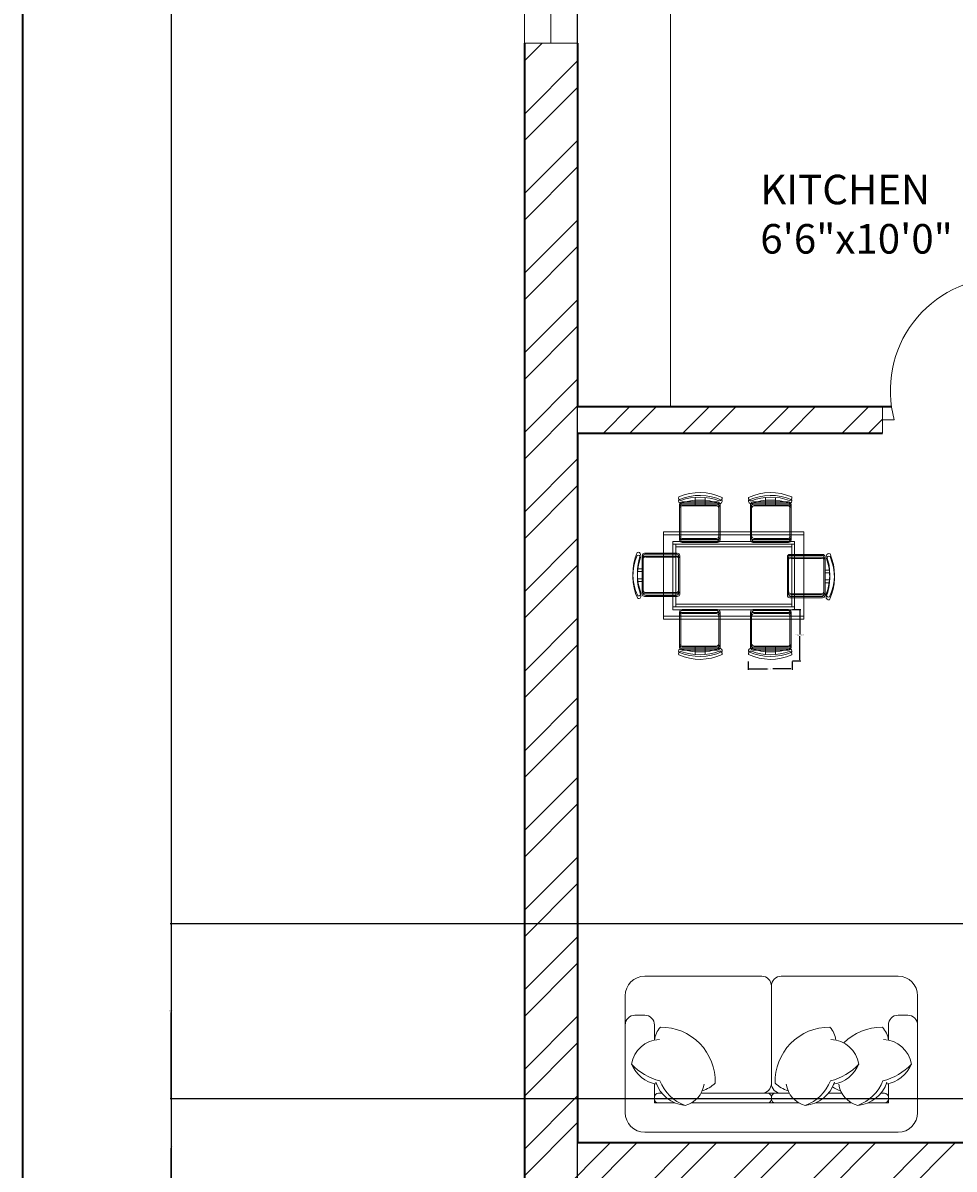
# Model space of a CAD drawing. Units: inches. Extents: x 2552 to 3217, y 1417 to 2737.
# Tile 16 of 25: x 2552 to 2710, y 2392 to 2585. Entities that reach past the tile are written whole.
import ezdxf

# ---------------------------------------------------------------- set-up
doc = ezdxf.new("R2010")
doc.units = ezdxf.units.IN
for name, color, linetype, lineweight in [('A-ANNO-DIMS', 2, 'Continuous', 18), ('A-ANNO-TTLB', 7, 'Continuous', 35), ('A-AREA-IDEN', 7, 'Continuous', 18), ('A-DOOR', 21, 'Continuous', 18), ('A-FLOR-CASE', 9, 'Continuous', 18), ('A-FURN', 8, 'Continuous', 13), ('A-GLAZ', 161, 'Continuous', 18), ('A-WALL', 7, 'Continuous', 35), ('A-WALL-PATT', 217, 'Continuous', 13)]:
    doc.layers.add(name, color=color, linetype=linetype, lineweight=lineweight)
doc.styles.get("Standard").update_dxf_attribs({"font": 'arial.ttf'})
doc.dimstyles.get("Standard").update_dxf_attribs({"dimtxt": 0.18, "dimasz": 0.18, "dimexe": 0.18, "dimexo": 0.0625, "dimgap": 0.09, "dimtad": 0, "dimtih": 1, "dimtoh": 1, "dimdec": 4, "dimzin": 0, "dimdsep": 46, "dimtxsty": 'Standard', "dimcen": 0.09, "dimadec": 0, "dimazin": 0, "dimtfac": 1, "dimtdec": 4, "dimtofl": 0, "dimtmove": 0, "dimatfit": 3, "dimfxl": 1, "dimtolj": 1, "dimtzin": 0, "dimarcsym": 0})

# ---------------------------------------------------------------- blocks, each defined once
blk = doc.blocks.new('TABLE-DINING-RECT')
for points in [[(0, 14.74), (23.77, 14.74), (23.77, 0.48), (0, 0.48)], [(0, 14.74), (23.77, 14.74), (23.77, 0.48), (0, 0.48)], [(0, 14.26), (23.77, 14.26), (23.77, 0), (0, 0)], [(0, 14.26), (23.77, 14.26), (23.77, 0), (0, 0)], [(1.58, 13.15), (22.19, 13.15), (22.19, 2.06), (1.58, 2.06)], [(1.58, 13.15), (22.19, 13.15), (22.19, 2.06), (1.58, 2.06)], [(1.58, 12.68), (22.19, 12.68), (22.19, 1.59), (1.58, 1.59)], [(1.58, 12.68), (22.19, 12.68), (22.19, 1.58), (1.58, 1.58)], [(2.06, 12.68), (21.71, 12.68), (21.71, 2.54), (2.06, 2.54)], [(2.06, 12.68), (21.71, 12.68), (21.71, 2.54), (2.06, 2.54)], [(2.06, 12.2), (21.71, 12.2), (21.71, 2.06), (2.06, 2.06)], [(2.06, 12.2), (21.71, 12.2), (21.71, 2.06), (2.06, 2.06)]]:
    blk.add_lwpolyline(points, close=True)
blk = doc.blocks.new('DINING-CHAIR-NORTH-EAST')
for points in [[(0.51, 7.05, -0.578392), (0.02, 7.59, -0.214524), (7.33, 7.69, -0.552014), (6.98, 7.1, 0.175809), (0.51, 7.05)], [(0.51, 7.05, -0.578392), (0.02, 7.59, -0.214524), (7.33, 7.69, -0.552014), (6.98, 7.1, 0.175809), (0.51, 7.05)], [(0.51, 6.58, -0.578392), (0.02, 7.12, -0.214524), (7.33, 7.22, -0.552014), (6.98, 6.63, 0.175809), (0.51, 6.58)], [(0.51, 6.58, -0.578392), (0.02, 7.12, -0.214524), (7.33, 7.22, -0.552014), (6.98, 6.63, 0.175809), (0.51, 6.58)], [(6.8, 6.84, -0.414214), (7.22, 6.42), (7.22, 0.9, -0.414214), (6.8, 0.48), (0.78, 0.48, -0.414214), (0.36, 0.9), (0.36, 6.42, -0.414214), (0.78, 6.84), (6.8, 6.84)], [(6.8, 6.84, -0.414214), (7.22, 6.42), (7.22, 0.9, -0.414214), (6.8, 0.48), (0.78, 0.48, -0.414214), (0.36, 0.9), (0.36, 6.42, -0.414214), (0.78, 6.84), (6.8, 6.84)], [(6.8, 6.37, -0.414214), (7.22, 5.95), (7.22, 0.42, -0.414214), (6.8, 0), (0.78, 0, -0.414214), (0.36, 0.42), (0.36, 5.95, -0.414214), (0.78, 6.37), (6.8, 6.37)], [(6.8, 6.37, -0.414214), (7.22, 5.95), (7.22, 0.42, -0.414214), (6.8, 0), (0.78, 0, -0.414214), (0.36, 0.42), (0.36, 5.95, -0.414214), (0.78, 6.37), (6.8, 6.37)], [(2.9, 6.84), (2.9, 7.6, 0.064759)], [(2.9, 6.84), (2.9, 7.6, 0.064759)], [(2.9, 6.37), (2.9, 7.13, 0.064759)], [(2.9, 6.37), (2.9, 7.13, 0.064759)]]:
    blk.add_lwpolyline(points, format="xyb")
for points in [[(6.79, 6.65), (0.97, 6.65, 0.414214), (0.55, 6.23), (0.55, 1.09, 0.414214), (0.97, 0.67), (6.79, 0.67, 0.512069), (7.03, 1.09), (7.03, 6.23, 0.512069)], [(6.79, 6.65), (0.97, 6.65, 0.414214), (0.55, 6.23), (0.55, 1.09, 0.414214), (0.97, 0.66), (6.79, 0.66, 0.512069), (7.03, 1.09), (7.03, 6.23, 0.512069)], [(6.79, 6.18), (0.97, 6.18, 0.414214), (0.55, 5.76), (0.55, 0.61, 0.414214), (0.97, 0.19), (6.79, 0.19, 0.512069), (7.03, 0.61), (7.03, 5.76, 0.512069)], [(6.79, 6.18), (0.97, 6.18, 0.414214), (0.55, 5.76), (0.55, 0.61, 0.414214), (0.97, 0.19), (6.79, 0.19, 0.512069), (7.03, 0.61), (7.03, 5.76, 0.512069)]]:
    blk.add_lwpolyline(points, format="xyb", close=True)
for points in [[(4.58, 7.62), (4.58, 6.84)], [(4.58, 7.62), (4.58, 6.84)], [(4.58, 7.14), (4.58, 6.37)], [(4.58, 7.14), (4.58, 6.37)]]:
    blk.add_lwpolyline(points)
blk = doc.blocks.new('DINING-CHAIR-SOUTH-WEST')
for points in [[(6.59, 2.06), (0.58, 2.06, -0.414214), (0.16, 2.48), (0.16, 8.01, -0.414214), (0.58, 8.43), (6.59, 8.43, -0.414214), (7.01, 8.01), (7.01, 2.48, -0.414214), (6.59, 2.06)], [(6.59, 2.06), (0.58, 2.06, -0.414214), (0.16, 2.48), (0.16, 8.01, -0.414214), (0.58, 8.43), (6.59, 8.43, -0.414214), (7.01, 8.01), (7.01, 2.48, -0.414214), (6.59, 2.06)], [(6.59, 1.58), (0.58, 1.58, -0.414214), (0.16, 2), (0.16, 7.53, -0.414214), (0.58, 7.95), (6.59, 7.95, -0.414214), (7.01, 7.53), (7.01, 2, -0.414214), (6.59, 1.58)], [(6.59, 1.58), (0.58, 1.58, -0.414214), (0.16, 2), (0.16, 7.53, -0.414214), (0.58, 7.95), (6.59, 7.95, -0.414214), (7.01, 7.53), (7.01, 2, -0.414214), (6.59, 1.58)], [(4.48, 2.06), (4.48, 1.3, 0.064759)], [(4.48, 2.06), (4.48, 1.3, 0.064759)], [(6.86, 1.85, -0.578392), (7.35, 1.31, -0.214524), (0.05, 1.21, -0.552014), (0.39, 1.8, 0.175809), (6.86, 1.85)], [(6.86, 1.85, -0.578392), (7.35, 1.31, -0.214524), (0.05, 1.21, -0.552014), (0.39, 1.8, 0.175809), (6.86, 1.85)], [(6.86, 1.37, -0.578392), (7.35, 0.83, -0.214524), (0.05, 0.74, -0.552014), (0.39, 1.32, 0.175809), (6.86, 1.37)], [(6.86, 1.37, -0.578392), (7.35, 0.83, -0.214524), (0.05, 0.74, -0.552014), (0.39, 1.32, 0.175809), (6.86, 1.37)], [(4.48, 1.58), (4.48, 0.82, 0.064759)], [(4.48, 1.58), (4.48, 0.82, 0.064759)]]:
    blk.add_lwpolyline(points, format="xyb")
for points in [[(0.58, 2.25), (6.4, 2.25, 0.414214), (6.82, 2.67), (6.82, 7.82, 0.414214), (6.4, 8.24), (0.58, 8.24, 0.512069), (0.35, 7.82), (0.35, 2.67, 0.512069)], [(0.58, 2.25), (6.4, 2.25, 0.414214), (6.82, 2.67), (6.82, 7.82, 0.414214), (6.4, 8.24), (0.58, 8.24, 0.512069), (0.35, 7.82), (0.35, 2.67, 0.512069)], [(0.58, 1.77), (6.4, 1.77, 0.414214), (6.82, 2.19), (6.82, 7.34, 0.414214), (6.4, 7.76), (0.58, 7.76, 0.512069), (0.35, 7.34), (0.35, 2.19, 0.512069)], [(0.58, 1.77), (6.4, 1.77, 0.414214), (6.82, 2.19), (6.82, 7.34, 0.414214), (6.4, 7.76), (0.58, 7.76, 0.512069), (0.35, 7.34), (0.35, 2.19, 0.512069)]]:
    blk.add_lwpolyline(points, format="xyb", close=True)
for points in [[(2.79, 1.28), (2.79, 2.06)], [(2.79, 1.28), (2.79, 2.06)], [(2.79, 0.81), (2.79, 1.58)], [(2.79, 0.81), (2.79, 1.58)]]:
    blk.add_lwpolyline(points)
blk = doc.blocks.new('DINING-CHAIR-SOUTH-EAST')
for points in [[(6.8, 2.06, 0.414214), (7.22, 2.48), (7.22, 8.01, 0.414214), (6.8, 8.43), (0.78, 8.43, 0.414214), (0.36, 8.01), (0.36, 2.48, 0.414214), (0.78, 2.06), (6.8, 2.06)], [(6.8, 2.06, 0.414214), (7.22, 2.48), (7.22, 8.01, 0.414214), (6.8, 8.43), (0.78, 8.43, 0.414214), (0.36, 8.01), (0.36, 2.48, 0.414214), (0.78, 2.06), (6.8, 2.06)], [(6.8, 1.58, 0.414214), (7.22, 2), (7.22, 7.53, 0.414214), (6.8, 7.95), (0.78, 7.95, 0.414214), (0.36, 7.53), (0.36, 2, 0.414214), (0.78, 1.58), (6.8, 1.58)], [(6.8, 1.58, 0.414214), (7.22, 2), (7.22, 7.53, 0.414214), (6.8, 7.95), (0.78, 7.95, 0.414214), (0.36, 7.53), (0.36, 2, 0.414214), (0.78, 1.58), (6.8, 1.58)], [(2.9, 2.06), (2.9, 1.3, -0.064759)], [(2.9, 2.06), (2.9, 1.3, -0.064759)], [(6.98, 1.8, -0.175809), (0.51, 1.85, 0.578392), (0.02, 1.31, 0.214524), (7.33, 1.21, 0.552014), (6.98, 1.8, -0.065079)], [(6.98, 1.8, -0.175809), (0.51, 1.85, 0.578392), (0.02, 1.31, 0.214524), (7.33, 1.21, 0.552014), (6.98, 1.8, -0.065079)], [(6.98, 1.32, -0.175809), (0.51, 1.37, 0.578392), (0.02, 0.83, 0.214524), (7.33, 0.74, 0.552014), (6.98, 1.32, -0.065079)], [(6.98, 1.32, -0.175809), (0.51, 1.37, 0.578392), (0.02, 0.83, 0.214524), (7.33, 0.74, 0.552014), (6.98, 1.32, -0.065079)], [(2.9, 1.58), (2.9, 0.82, -0.064759)], [(2.9, 1.58), (2.9, 0.82, -0.064759)]]:
    blk.add_lwpolyline(points, format="xyb")
for points in [[(6.79, 2.25), (0.97, 2.25, -0.414214), (0.55, 2.67), (0.55, 7.82, -0.414214), (0.97, 8.24), (6.79, 8.24, -0.512069), (7.03, 7.82), (7.03, 2.67, -0.512069)], [(6.79, 2.25), (0.97, 2.25, -0.414214), (0.55, 2.67), (0.55, 7.82, -0.414214), (0.97, 8.24), (6.79, 8.24, -0.512069), (7.03, 7.82), (7.03, 2.67, -0.512069)], [(6.79, 1.77), (0.97, 1.77, -0.414214), (0.55, 2.19), (0.55, 7.34, -0.414214), (0.97, 7.76), (6.79, 7.76, -0.512069), (7.03, 7.34), (7.03, 2.19, -0.512069)], [(6.79, 1.77), (0.97, 1.77, -0.414214), (0.55, 2.19), (0.55, 7.34, -0.414214), (0.97, 7.76), (6.79, 7.76, -0.512069), (7.03, 7.34), (7.03, 2.19, -0.512069)]]:
    blk.add_lwpolyline(points, format="xyb", close=True)
for points in [[(4.58, 1.28), (4.58, 2.06)], [(4.58, 1.28), (4.58, 2.06)], [(4.58, 0.81), (4.58, 1.58)], [(4.58, 0.81), (4.58, 1.58)]]:
    blk.add_lwpolyline(points)
blk = doc.blocks.new('WIN-36')
for p, q in [((4.5, 36), (0, 36)), ((0, 36), (9, 36)), ((0, 36), (0, 0)), ((4.5, 0), (4.5, 36)), ((9, 36), (9, 0)), ((0, 0), (9, 0)), ((9, 0), (4.5, 0))]:
    blk.add_line(p, q)
blk = doc.blocks.new('*D29')
at = {"layer": 'A-ANNO-DIMS', "color": 0, "lineweight": -2, "transparency": 16777216}
for p, q in [((2682.71, 2486.17), (2684.14, 2486.17)), ((2683.96, 2485.99), (2683.96, 2482)), ((2683.96, 2477.65), (2683.96, 2481.64)), ((2682.71, 2477.47), (2684.14, 2477.47))]:
    blk.add_line(p, q, dxfattribs=at)
at = {"layer": 'A-ANNO-DIMS', "color": 0, "transparency": 16777216}
for points in [[(2683.93, 2485.99), (2683.99, 2485.99), (2683.96, 2486.17)], [(2683.93, 2477.65), (2683.99, 2477.65), (2683.96, 2477.47)]]:
    blk.add_solid(points, dxfattribs=at)
at = {"layer": 'Defpoints', "color": 0, "transparency": 16777216}
for p in [(2682.65, 2486.17), (2683.96, 2486.17), (2682.65, 2477.47)]:
    blk.add_point(p, dxfattribs=at)
at = {"layer": 'A-ANNO-DIMS', "color": 0, "transparency": 16777216, "insert": (2683.96, 2481.82), "char_height": 0.18, "attachment_point": 5}
blk.add_mtext('\\A1;CHAIR 9 TYP.', dxfattribs=at)
blk = doc.blocks.new('*D30')
at = {"layer": 'A-ANNO-DIMS', "color": 0, "lineweight": -2, "transparency": 16777216}
for p, q in [((2675.23, 2477.4), (2675.23, 2475.98)), ((2675.41, 2476.16), (2678.49, 2476.16)), ((2682.47, 2476.16), (2679.4, 2476.16)), ((2682.65, 2477.4), (2682.65, 2475.98))]:
    blk.add_line(p, q, dxfattribs=at)
at = {"layer": 'A-ANNO-DIMS', "color": 0, "transparency": 16777216}
for points in [[(2675.41, 2476.19), (2675.41, 2476.13), (2675.23, 2476.16)], [(2682.47, 2476.19), (2682.47, 2476.13), (2682.65, 2476.16)]]:
    blk.add_solid(points, dxfattribs=at)
at = {"layer": 'Defpoints', "color": 0, "transparency": 16777216}
for p in [(2675.23, 2477.47), (2682.65, 2477.47), (2682.65, 2476.16)]:
    blk.add_point(p, dxfattribs=at)
at = {"layer": 'A-ANNO-DIMS', "color": 0, "transparency": 16777216, "insert": (2678.94, 2476.16), "char_height": 0.18, "attachment_point": 5}
blk.add_mtext('\\A1;7 TYP.', dxfattribs=at)
blk = doc.blocks.new('*D50')
at = {"layer": 'A-ANNO-DIMS', "color": 0, "lineweight": -2, "transparency": 16777216}
for p, q in [((2637.29, 2649.51), (2577.37, 2649.51)), ((2577.55, 2649.33), (2577.55, 2096.19)), ((2577.55, 1542.69), (2577.55, 2095.83)), ((2637.29, 1542.51), (2577.37, 1542.51))]:
    blk.add_line(p, q, dxfattribs=at)
at = {"layer": 'A-ANNO-DIMS', "color": 0, "transparency": 16777216}
for points in [[(2577.52, 2649.33), (2577.58, 2649.33), (2577.55, 2649.51)], [(2577.52, 1542.69), (2577.58, 1542.69), (2577.55, 1542.51)]]:
    blk.add_solid(points, dxfattribs=at)
at = {"layer": 'Defpoints', "color": 0, "transparency": 16777216}
for p in [(2577.55, 2649.51), (2637.35, 2649.51), (2637.35, 1542.51)]:
    blk.add_point(p, dxfattribs=at)
at = {"layer": 'A-ANNO-DIMS', "color": 0, "transparency": 16777216, "insert": (2577.55, 2096.01), "char_height": 0.18, "attachment_point": 5}
blk.add_mtext('\\A1;1107', dxfattribs=at)
blk = doc.blocks.new('*D55')
at = {"layer": 'A-ANNO-DIMS', "color": 0, "lineweight": -2, "transparency": 16777216}
for p, q in [((2908.79, 2433), (2577.37, 2433)), ((2577.55, 2432.82), (2577.55, 2418.39)), ((2577.55, 2403.59), (2577.55, 2418.02)), ((2908.79, 2403.41), (2577.37, 2403.41))]:
    blk.add_line(p, q, dxfattribs=at)
at = {"layer": 'A-ANNO-DIMS', "color": 0, "transparency": 16777216}
for points in [[(2577.52, 2432.82), (2577.58, 2432.82), (2577.55, 2433)], [(2577.52, 2403.59), (2577.58, 2403.59), (2577.55, 2403.41)]]:
    blk.add_solid(points, dxfattribs=at)
at = {"layer": 'Defpoints', "color": 0, "transparency": 16777216}
for p in [(2577.55, 2433), (2908.85, 2433), (2908.85, 2403.41)]:
    blk.add_point(p, dxfattribs=at)
at = {"layer": 'A-ANNO-DIMS', "color": 0, "transparency": 16777216, "insert": (2577.55, 2418.21), "char_height": 0.18, "attachment_point": 5}
blk.add_mtext('\\A1;29.59', dxfattribs=at)
blk = doc.blocks.new('*D64')
at = {"layer": 'A-ANNO-DIMS', "color": 0, "lineweight": -2, "transparency": 16777216}
for p, q in [((2646.35, 1551.58), (2646.35, 2709.49)), ((2646.53, 2709.31), (2802.77, 2709.31)), ((2959.93, 2709.31), (2803.69, 2709.31)), ((2960.11, 1551.58), (2960.11, 2709.49))]:
    blk.add_line(p, q, dxfattribs=at)
at = {"layer": 'A-ANNO-DIMS', "color": 0, "transparency": 16777216}
for points in [[(2646.53, 2709.34), (2646.53, 2709.28), (2646.35, 2709.31)], [(2959.93, 2709.34), (2959.93, 2709.28), (2960.11, 2709.31)]]:
    blk.add_solid(points, dxfattribs=at)
at = {"layer": 'Defpoints', "color": 0, "transparency": 16777216}
for p in [(2960.11, 2709.31), (2646.35, 1551.51), (2960.11, 1551.51)]:
    blk.add_point(p, dxfattribs=at)
at = {"layer": 'A-ANNO-DIMS', "color": 0, "transparency": 16777216, "insert": (2803.23, 2709.31), "char_height": 0.18, "attachment_point": 5}
blk.add_mtext('\\A1;313.76', dxfattribs=at)
blk = doc.blocks.new('*D69')
at = {"layer": 'A-ANNO-DIMS', "color": 0, "lineweight": -2, "transparency": 16777216}
for p, q in [((2908.79, 2403.41), (2577.37, 2403.41)), ((2577.55, 2403.23), (2577.55, 2395.39)), ((2577.55, 2387.19), (2577.55, 2395.03)), ((2917.79, 2387.01), (2577.37, 2387.01))]:
    blk.add_line(p, q, dxfattribs=at)
at = {"layer": 'A-ANNO-DIMS', "color": 0, "transparency": 16777216}
for points in [[(2577.52, 2403.23), (2577.58, 2403.23), (2577.55, 2403.41)], [(2577.52, 2387.19), (2577.58, 2387.19), (2577.55, 2387.01)]]:
    blk.add_solid(points, dxfattribs=at)
at = {"layer": 'Defpoints', "color": 0, "transparency": 16777216}
for p in [(2577.55, 2403.41), (2908.85, 2403.41), (2917.85, 2387.01)]:
    blk.add_point(p, dxfattribs=at)
at = {"layer": 'A-ANNO-DIMS', "color": 0, "transparency": 16777216, "insert": (2577.55, 2395.21), "char_height": 0.18, "attachment_point": 5}
blk.add_mtext('\\A1;16.4', dxfattribs=at)

msp = doc.modelspace()

# ---------------------------------------------------------------- hatches: boundary and pattern name
at = {"layer": 'A-WALL-PATT'}
h = msp.add_hatch(dxfattribs=at)
h.set_pattern_fill('ANSI32', color=256)
h.paths.add_polyline_path([(2756.676, 2649.5125), (2637.3535, 2649.5125), (2637.3535, 2617.9626), (2641.8535, 2617.9626), (2646.3535, 2617.9626), (2646.3535, 2640.5125), (2724.3535, 2640.5125), (2724.3535, 2520.5125), (2720.299, 2520.5125), (2720.299, 2516.0125), (2733.4075, 2516.0125), (2733.4075, 2518.2213), (2733.4075, 2520.5125), (2728.8535, 2520.5125), (2728.8535, 2640.5125), (2756.676, 2640.5125)])
h.paths.add_polyline_path([(2848.8535, 2649.5125), (2804.676, 2649.5125), (2804.676, 2640.5125), (2839.8535, 2640.5125), (2839.8535, 2598.3517), (2848.8535, 2598.3517)])
h.paths.add_polyline_path([(2646.3535, 2516.0125), (2697.9593, 2516.0125), (2697.9593, 2518.2625), (2697.9593, 2520.5125), (2646.3535, 2520.5125), (2646.3535, 2581.9626), (2637.3535, 2581.9626), (2637.3535, 2364.3298), (2646.3535, 2364.3298), (2646.3535, 2387.0125), (2724.3535, 2387.0125), (2724.3535, 2267.0125), (2721.0443, 2267.0125), (2721.0443, 2262.5125), (2733.7854, 2262.5125), (2733.7854, 2264.7625), (2733.7854, 2267.0125), (2728.8535, 2267.0125), (2728.8535, 2387.0125), (2839.8535, 2387.0125), (2839.8535, 2363.8387), (2848.8535, 2363.8387), (2848.8535, 2403.7415), (2844.3535, 2403.7415), (2839.8535, 2403.7415), (2839.8535, 2396.0125), (2646.3535, 2396.0125)])
h.paths.add_polyline_path([(2848.8535, 2550.3517), (2844.3535, 2550.3517), (2839.8535, 2550.3517), (2839.8535, 2520.5125), (2801.9195, 2520.5125), (2801.9195, 2518.2625), (2801.9195, 2516.0125), (2839.8535, 2516.0125), (2839.8535, 2507.5813), (2848.8535, 2507.5813)], flags=17)
h.paths.add_polyline_path([(2848.8535, 2483.5813), (2844.3535, 2483.5813), (2839.8535, 2483.5813), (2839.8535, 2468.0125), (2773.8535, 2468.0125), (2773.8535, 2516.0125), (2778.1336, 2516.0125), (2778.1336, 2520.5125), (2766.696, 2520.5125), (2766.696, 2518.2625), (2766.696, 2516.0125), (2769.3535, 2516.0125), (2769.3535, 2463.5125), (2839.8535, 2463.5125), (2839.8535, 2431.0782), (2848.8535, 2431.0782)], flags=17)
h.paths.add_polyline_path([(2917.8535, 2569.2764), (2913.3535, 2569.2764), (2908.8535, 2569.2764), (2908.8535, 2433.001), (2917.8535, 2433.001), (2917.8535, 2516.0125), (2967.486, 2516.0125), (2967.486, 2520.5125), (2917.8535, 2520.5125)])
h.paths.add_polyline_path([(3000.3535, 2640.5125), (2995.8535, 2640.5125), (2995.8535, 2520.5125), (2990.688, 2520.5125), (2990.688, 2516.0125), (3004.0844, 2516.0125), (3004.0844, 2518.2625), (3004.0844, 2520.5125), (3000.3535, 2520.5125)])
h.paths.add_polyline_path([(3120.3535, 2561.3689), (3115.8535, 2561.3689), (3111.3535, 2561.3689), (3111.3535, 2520.5125), (3070.9814, 2520.5125), (3070.9814, 2518.2625), (3070.9814, 2516.0125), (3111.3535, 2516.0125), (3111.3535, 2505.1841), (3120.3535, 2505.1841)])
h.paths.add_polyline_path([(3120.3535, 2481.1841), (3115.8535, 2481.1841), (3111.3535, 2481.1841), (3111.3535, 2468.0125), (3045.3535, 2468.0125), (3045.3535, 2516.0125), (3048.9787, 2516.0125), (3048.9787, 2520.5125), (3036.3395, 2520.5125), (3036.3395, 2516.0125), (3040.8535, 2516.0125), (3040.8535, 2463.5125), (3111.3535, 2463.5125), (3111.3535, 2396.0125), (2917.8535, 2396.0125), (2917.8535, 2403.4124), (2913.3535, 2403.4124), (2908.8535, 2403.4124), (2908.8535, 2182.5756), (2917.8535, 2182.5756), (2917.8535, 2262.5125), (2968.001, 2262.5125), (2968.001, 2264.7625), (2968.001, 2267.0125), (2917.8535, 2267.0125), (2917.8535, 2387.0125), (3111.3535, 2387.0125), (3111.3535, 2352.2435), (3120.3535, 2352.2435)])
h.paths.add_polyline_path([(3120.3535, 2304.2435), (3115.8535, 2304.2435), (3111.3535, 2304.2435), (3111.3535, 2267.0125), (3073.8616, 2267.0125), (3073.8616, 2264.7625), (3073.8616, 2262.5125), (3111.3535, 2262.5125), (3111.3535, 2252.376), (3120.3535, 2252.376)], flags=17)
h.paths.add_polyline_path([(3120.3535, 2228.376), (3115.8535, 2228.376), (3111.3535, 2228.376), (3111.3535, 2214.5125), (3045.3535, 2214.5125), (3045.3535, 2262.5125), (3049.3096, 2262.5125), (3049.3096, 2267.0125), (3035.0125, 2267.0125), (3035.0125, 2262.5125), (3040.8535, 2262.5125), (3040.8535, 2210.0125), (3111.3535, 2210.0125), (3111.3535, 2142.5125), (2917.8535, 2142.5125), (2917.8535, 2150.2408), (2913.3535, 2150.2408), (2908.8535, 2150.2408), (2908.8535, 1924.9905), (2917.8535, 1924.9905), (2917.8535, 2009.0125), (2971.959, 2009.0125), (2971.959, 2011.2625), (2971.959, 2013.5125), (2917.8535, 2013.5125), (2917.8535, 2133.5125), (2995.8535, 2133.5125), (2995.8535, 2013.5125), (2992.1797, 2013.5125), (2992.1797, 2009.0125), (3004.3344, 2009.0125), (3004.3344, 2011.2625), (3004.3344, 2013.5125), (3000.3535, 2013.5125), (3000.3535, 2133.5125), (3111.3535, 2133.5125), (3111.3535, 2115.0291), (3120.3535, 2115.0291)])
h.paths.add_polyline_path([(3000.3535, 2387.0125), (2995.8535, 2387.0125), (2995.8535, 2267.0125), (2991.3326, 2267.0125), (2991.3326, 2262.5125), (3004.1044, 2262.5125), (3004.1044, 2264.7625), (3004.1044, 2267.0125), (3000.3535, 2267.0125)], flags=17)
h.paths.add_polyline_path([(3120.3535, 1973.2388), (3115.8535, 1973.2388), (3111.3535, 1973.2388), (3111.3535, 1961.0125), (3045.3535, 1961.0125), (3045.3535, 2009.0125), (3048.9101, 2009.0125), (3048.9101, 2013.5125), (3037.105, 2013.5125), (3037.105, 2011.2625), (3037.105, 2009.0125), (3040.8535, 2009.0125), (3040.8535, 1956.5125), (3111.3535, 1956.5125), (3111.3535, 1889.0125), (2917.8535, 1889.0125), (2917.8535, 1895.7215), (2913.3535, 1895.7215), (2908.8535, 1895.7215), (2908.8535, 1844.2217), (2917.8535, 1844.2217), (2917.8535, 1880.0125), (3111.3535, 1880.0125), (3111.3535, 1846.9541), (3120.3535, 1846.9541)])
h.paths.add_polyline_path([(3120.3535, 2067.0291), (3111.3535, 2067.0291), (3111.3535, 2013.5125), (3071.3001, 2013.5125), (3071.3001, 2009.0125), (3111.3535, 2009.0125), (3111.3535, 1997.2388), (3120.3535, 1997.2388)], flags=0)
h.paths.add_polyline_path([(3120.3535, 1798.9541), (3115.8535, 1798.9541), (3111.3535, 1798.9541), (3111.3535, 1760.0125), (3071.2497, 1760.0125), (3071.2497, 1757.7625), (3071.2497, 1755.5125), (3111.3535, 1755.5125), (3111.3535, 1746.162), (3120.3535, 1746.2478)])
h.paths.add_polyline_path([(3120.3535, 1722.2049), (3111.3535, 1722.2049), (3111.3535, 1707.5125), (3045.3535, 1707.5125), (3045.3535, 1755.5125), (3048.6624, 1755.5125), (3048.6624, 1760.0125), (3035.3703, 1760.0125), (3035.3703, 1755.5125), (3040.8535, 1755.5125), (3040.8535, 1703.0125), (3111.3535, 1703.0125), (3111.3535, 1635.5125), (2917.8535, 1635.5125), (2917.8535, 1643.1366), (2913.3535, 1643.1366), (2908.8535, 1643.1366), (2908.8535, 1626.5125), (3120.3535, 1626.5125)])
h.paths.add_polyline_path([(2917.8535, 1755.5125), (2973.2287, 1755.5125), (2973.2287, 1757.7625), (2973.2287, 1760.0125), (2917.8535, 1760.0125), (2917.8535, 1808.2217), (2913.3535, 1808.2217), (2908.8535, 1808.2217), (2908.8535, 1676.1665), (2917.8535, 1676.1665)])
h.paths.add_polyline_path([(3000.3535, 1880.0125), (2995.8535, 1880.0125), (2995.8535, 1760.0125), (2992.9329, 1760.0125), (2992.9329, 1755.5125), (3003.8766, 1755.5125), (3003.8766, 1757.7625), (3003.8766, 1760.0125), (3000.3535, 1760.0125)])
h.paths.add_polyline_path([(2848.8535, 1896.6971), (2844.3535, 1896.6971), (2839.8535, 1896.6971), (2839.8535, 1889.0125), (2646.3535, 1889.0125), (2646.3535, 2009.0125), (2700.5253, 2009.0125), (2700.5253, 2011.2625), (2700.5253, 2013.5125), (2646.3535, 2013.5125), (2646.3535, 2053.1812), (2641.8535, 2053.1812), (2637.3535, 2053.1812), (2637.3535, 1836.254), (2646.3535, 1836.254), (2646.3535, 1880.0125), (2724.3535, 1880.0125), (2724.3535, 1760.0125), (2721.2473, 1760.0125), (2721.2473, 1755.5125), (2731.9187, 1755.5125), (2731.9187, 1757.7625), (2731.9187, 1760.0125), (2728.8535, 1760.0125), (2728.8535, 1880.0125), (2839.8535, 1880.0125), (2839.8535, 1840.3813), (2848.8535, 1840.3813)])
h.paths.add_polyline_path([(2848.8535, 1792.3813), (2844.3535, 1792.3813), (2839.8535, 1792.3813), (2839.8535, 1760.0125), (2797.8845, 1760.0125), (2797.8845, 1755.5125), (2839.8535, 1755.5125), (2839.8535, 1743.3688), (2844.3535, 1743.3688), (2848.8535, 1743.3688)], flags=0)
h.paths.add_polyline_path([(2848.8535, 1719.3688), (2844.3535, 1719.3688), (2839.8535, 1719.3688), (2839.8535, 1707.5125), (2773.8535, 1707.5125), (2773.8535, 1755.5125), (2777.716, 1755.5125), (2777.716, 1760.0125), (2760.9247, 1760.0125), (2760.9247, 1757.9721), (2760.9247, 1755.5125), (2769.3535, 1755.5125), (2769.3535, 1703.0125), (2839.8535, 1703.0125), (2839.8535, 1673.0277), (2848.8535, 1672.9407)], flags=0)
h.paths.add_polyline_path([(2646.3535, 1755.5125), (2702.9171, 1755.5125), (2702.9171, 1757.7625), (2702.9171, 1760.0125), (2646.3535, 1760.0125), (2646.3535, 1800.254), (2641.8535, 1800.254), (2637.3535, 1800.254), (2637.3535, 1626.5125), (2848.8535, 1626.5125), (2848.8535, 1643.1187), (2844.3535, 1643.1187), (2839.8535, 1643.1187), (2839.8535, 1635.5125), (2646.3535, 1635.5125)])
h.paths.add_polyline_path([(2848.8535, 2148.8427), (2844.3535, 2148.8427), (2839.8535, 2148.8427), (2839.8535, 2142.5125), (2646.3535, 2142.5125), (2646.3535, 2262.5125), (2701.3562, 2262.5125), (2701.3562, 2264.7625), (2701.3562, 2267.0125), (2646.3535, 2267.0125), (2646.3535, 2328.3298), (2637.3535, 2328.3298), (2637.3535, 2089.1812), (2646.3535, 2089.1812), (2646.3535, 2133.5125), (2839.8535, 2133.5125), (2839.8535, 2097.5966), (2848.8535, 2097.5966)])
h.paths.add_polyline_path([(2728.8535, 2133.5125), (2724.3535, 2133.5125), (2724.3535, 2013.5125), (2719.6039, 2013.5125), (2719.6039, 2009.0125), (2732.5784, 2009.0125), (2732.5784, 2011.2625), (2732.5784, 2013.5125), (2728.8535, 2013.5125)])
h.paths.add_polyline_path([(2848.8535, 1970.0557), (2844.3535, 1970.0557), (2839.8535, 1970.0557), (2839.8535, 1961.0125), (2773.8535, 1961.0125), (2773.8535, 2009.0125), (2777.3388, 2009.0125), (2777.3388, 2013.5125), (2764.7681, 2013.5125), (2764.7681, 2009.0125), (2769.3535, 2009.0125), (2769.3535, 1956.5125), (2839.8535, 1956.5125), (2839.8535, 1924.7199), (2848.8535, 1924.7199)], flags=17)
h.paths.add_polyline_path([(2848.8535, 2049.5966), (2844.3535, 2049.5966), (2839.8535, 2049.5966), (2839.8535, 2013.5125), (2798.198, 2013.5125), (2798.198, 2011.2625), (2798.198, 2009.0125), (2839.8535, 2009.0125), (2839.8535, 1994.0557), (2848.8535, 1994.0557)], flags=17)
h.paths.add_polyline_path([(2848.8535, 2315.8387), (2839.8535, 2315.8387), (2839.8535, 2267.0125), (2799.3375, 2267.0125), (2799.3375, 2264.7625), (2799.3375, 2262.5125), (2839.8535, 2262.5125), (2839.8535, 2253.2843), (2848.8535, 2253.2843)], flags=17)
h.paths.add_polyline_path([(2848.8535, 2229.2843), (2839.8535, 2229.2843), (2839.8535, 2177.6936), (2848.8535, 2177.6936)], flags=17)
h.paths.add_polyline_path([(2839.8535, 2214.5125), (2773.8535, 2214.5125), (2773.8535, 2262.5125), (2777.6984, 2262.5125), (2777.6984, 2267.0125), (2763.8226, 2267.0125), (2763.8226, 2262.5125), (2769.3535, 2262.5125), (2769.3535, 2210.0125), (2839.8535, 2210.0125)], flags=17)
h.paths.add_polyline_path([(3050.32, 2520.2817), (3088.9114, 2520.2817), (3088.9114, 2538.939), (3050.32, 2538.939)], flags=9)

# ---------------------------------------------------------------- linework, layer by layer
at = {"layer": 'A-ANNO-TTLB'}
msp.add_lwpolyline([(2552.473, 2736.5692), (3216.7862, 2736.5692), (3216.7862, 1416.6914), (2552.473, 1416.6914)], close=True, dxfattribs=at)
at = {"layer": 'A-DOOR'}
for p, q in [((2697.9593, 2520.5125), (2697.9593, 2516.0125)), ((2697.9593, 2516.0125), (2697.9593, 2518.2625)), ((2697.9593, 2518.2625), (2699.9593, 2518.2625))]:
    msp.add_line(p, q, dxfattribs=at)
msp.add_arc((2718.299, 2523.2554), 19.0071, 90, 195.22938, dxfattribs=at)
at = {"layer": 'A-FLOR-CASE'}
for q in [(2662.102, 2623.7542), (2662.102, 2520.5125)]:
    msp.add_line((2662.102, 2520.5125), q, dxfattribs=at)
at = {"layer": 'A-FURN'}
for points in [[(2663.8448, 2504.6312, -0.17580919), (2670.3193, 2504.5822, 0.57839206), (2670.8097, 2505.1215, 0.21452438), (2663.5015, 2505.2196, 0.55201397), (2663.8448, 2504.6312, -0.06507904)], [(2663.8448, 2504.631, -0.17580919), (2670.3193, 2504.5819, 0.57839206), (2670.8098, 2505.1213, 0.21452438), (2663.5015, 2505.2193, 0.55201397), (2663.8448, 2504.631, -0.06507904)], [(2663.8448, 2504.1558, -0.17580919), (2670.3193, 2504.1068, 0.57839206), (2670.8097, 2504.6461, 0.21452438), (2663.5015, 2504.7442, 0.55201397), (2663.8448, 2504.1558, -0.06507904)], [(2663.8448, 2504.1556, -0.17580919), (2670.3193, 2504.1065, 0.57839206), (2670.8098, 2504.6459, 0.21452438), (2663.5015, 2504.7439, 0.55201397), (2663.8448, 2504.1556, -0.06507904)], [(2670.0446, 2504.3714), (2664.0339, 2504.3714, 0.41421356), (2663.6134, 2503.9509), (2663.6134, 2498.4242, 0.41421356), (2664.0339, 2498.0037), (2670.0446, 2498.0037, 0.41421356), (2670.4651, 2498.4242), (2670.4651, 2503.9509, 0.41421356), (2670.0446, 2504.3714)], [(2670.0446, 2504.3711), (2664.0339, 2504.3711, 0.41421356), (2663.6134, 2503.9506), (2663.6134, 2498.4239, 0.41421356), (2664.0339, 2498.0034), (2670.0446, 2498.0034, 0.41421356), (2670.4651, 2498.4239), (2670.4651, 2503.9506, 0.41421356), (2670.0446, 2504.3711)], [(2670.0446, 2503.896), (2664.0339, 2503.896, 0.41421356), (2663.6134, 2503.4754), (2663.6134, 2497.9487, 0.41421356), (2664.0339, 2497.5282), (2670.0446, 2497.5282, 0.41421356), (2670.4651, 2497.9487), (2670.4651, 2503.4754, 0.41421356), (2670.0446, 2503.896)], [(2670.0446, 2503.8957), (2664.0339, 2503.8957, 0.41421356), (2663.6134, 2503.4752), (2663.6134, 2497.9485, 0.41421356), (2664.0339, 2497.528), (2670.0446, 2497.528, 0.41421356), (2670.4651, 2497.9485), (2670.4651, 2503.4752, 0.41421356), (2670.0446, 2503.8957)], [(2667.9333, 2504.3714), (2667.9333, 2505.1315, -0.06475861)], [(2667.9333, 2504.3711), (2667.9333, 2505.1313, -0.06475861)], [(2667.9333, 2503.896), (2667.9333, 2504.6561, -0.06475861)], [(2667.9333, 2503.8957), (2667.9333, 2504.6559, -0.06475861)], [(2657.0713, 2488.9964, -0.57839206), (2656.532, 2488.5059, -0.21452438), (2656.4339, 2495.8142, -0.55201397), (2657.0223, 2495.4709, 0.17580937), (2657.0713, 2488.9964)], [(2657.0713, 2488.9962, -0.57839206), (2656.532, 2488.5057, -0.21452438), (2656.4339, 2495.8139, -0.55201397), (2657.0223, 2495.4706, 0.17580937), (2657.0713, 2488.9961)], [(2657.2821, 2495.2817, -0.41421356), (2657.7026, 2495.7023), (2663.2293, 2495.7023, -0.41421356), (2663.6498, 2495.2817), (2663.6498, 2489.2711, -0.41421356), (2663.2293, 2488.8506), (2657.7026, 2488.8506, -0.41421356), (2657.2821, 2489.2711), (2657.2821, 2495.2817)], [(2657.2821, 2495.2815, -0.41421356), (2657.7026, 2495.702), (2663.2293, 2495.702, -0.41421356), (2663.6498, 2495.2815), (2663.6498, 2489.2708, -0.41421356), (2663.2293, 2488.8503), (2657.7026, 2488.8503, -0.41421356), (2657.2821, 2489.2708), (2657.2821, 2495.2815)], [(2688.4941, 2495.265, -0.17580919), (2688.445, 2488.7905, 0.57839206), (2688.9844, 2488.3001, 0.21452438), (2689.0824, 2495.6083, 0.55201397), (2688.4941, 2495.265, -0.06507904)], [(2688.4941, 2495.2647, -0.17580919), (2688.445, 2488.7903, 0.57839206), (2688.9844, 2488.2998, 0.21452438), (2689.0824, 2495.6081, 0.55201397), (2688.4941, 2495.2647, -0.06507904)], [(2657.0713, 2488.521, -0.57839206), (2656.532, 2488.0305, -0.21452438), (2656.4339, 2495.3388, -0.55201397), (2657.0223, 2494.9954, 0.17580937), (2657.0713, 2488.521)], [(2657.0713, 2488.5207, -0.57839206), (2656.532, 2488.0302, -0.21452438), (2656.4339, 2495.3385, -0.55201397), (2657.0223, 2494.9952, 0.17580937), (2657.0713, 2488.5207)], [(2657.2821, 2494.8063, -0.41421356), (2657.7026, 2495.2268), (2663.2293, 2495.2268, -0.41421356), (2663.6498, 2494.8063), (2663.6498, 2488.7957, -0.41421356), (2663.2293, 2488.3752), (2657.7026, 2488.3752, -0.41421356), (2657.2821, 2488.7957), (2657.2821, 2494.8063)], [(2657.2821, 2494.8061, -0.41421356), (2657.7026, 2495.2266), (2663.2293, 2495.2266, -0.41421356), (2663.6498, 2494.8061), (2663.6498, 2488.7954, -0.41421356), (2663.2293, 2488.3749), (2657.7026, 2488.3749, -0.41421356), (2657.2821, 2488.7954), (2657.2821, 2494.8061)], [(2688.2342, 2495.0759, 0.41421356), (2687.8137, 2495.4964), (2682.287, 2495.4964, 0.41421356), (2681.8665, 2495.0759), (2681.8665, 2489.0652, 0.41421356), (2682.287, 2488.6447), (2687.8137, 2488.6447, 0.41421356), (2688.2342, 2489.0652), (2688.2342, 2495.0759)], [(2688.2342, 2495.0756, 0.41421356), (2687.8137, 2495.4962), (2682.287, 2495.4962, 0.41421356), (2681.8665, 2495.0756), (2681.8665, 2489.065, 0.41421356), (2682.287, 2488.6445), (2687.8137, 2488.6445, 0.41421356), (2688.2342, 2489.065), (2688.2342, 2495.0756)], [(2688.2342, 2494.6005, 0.41421356), (2687.8137, 2495.021), (2682.287, 2495.021, 0.41421356), (2681.8665, 2494.6005), (2681.8665, 2488.5898, 0.41421356), (2682.287, 2488.1693), (2687.8137, 2488.1693, 0.41421356), (2688.2342, 2488.5898), (2688.2342, 2494.6005)], [(2688.2342, 2494.6002, 0.41421356), (2687.8137, 2495.0207), (2682.287, 2495.0207, 0.41421356), (2681.8665, 2494.6002), (2681.8665, 2488.5896, 0.41421356), (2682.287, 2488.1691), (2687.8137, 2488.1691, 0.41421356), (2688.2342, 2488.5896), (2688.2342, 2494.6002)], [(2688.4941, 2494.7896, -0.17580919), (2688.445, 2488.3151, 0.57839206), (2688.9844, 2487.8246, 0.21452438), (2689.0824, 2495.1329, 0.55201397), (2688.4941, 2494.7896, -0.06507904)], [(2688.4941, 2494.7893, -0.17580919), (2688.445, 2488.3149, 0.57839206), (2688.9844, 2487.8244, 0.21452438), (2689.0824, 2495.1327, 0.55201397), (2688.4941, 2494.7893, -0.06507904)], [(2657.2821, 2491.3823), (2656.5219, 2491.3823, 0.06475861)], [(2657.2821, 2490.9069), (2656.5219, 2490.9069, 0.06475861)], [(2657.2821, 2491.3821), (2656.522, 2491.3821, 0.06475861)], [(2657.2821, 2490.9067), (2656.522, 2490.9067, 0.06475861)], [(2688.2342, 2491.1765), (2688.9944, 2491.1765, -0.06475861)], [(2688.2342, 2491.1762), (2688.9944, 2491.1762, -0.06475861)], [(2688.2342, 2490.7011), (2688.9944, 2490.7011, -0.06475861)], [(2688.2342, 2490.7008), (2688.9944, 2490.7008, -0.06475861)], [(2677.5108, 2404.3449, 0.41421356), (2679.1604, 2405.9945), (2679.1604, 2422.4901, 0.41421356)], [(2680.8099, 2404.3449, -0.41421356), (2679.1604, 2405.9945), (2679.1604, 2422.4901, -0.41421356)], [(2654.4169, 2415.8918, -0.41421356), (2656.0665, 2417.5414), (2657.716, 2417.5414, -0.41421356), (2659.3656, 2415.8918), (2659.3656, 2413.3361)], [(2698.9551, 2413.3361), (2698.9551, 2415.8918, -0.41421356), (2700.6047, 2417.5414), (2702.2542, 2417.5414, -0.41421356), (2703.9038, 2415.8918)], [(2659.362, 2413.3353, -0.16554063), (2660.3825, 2415.5149, -0.42598917), (2669.6467, 2406.0651, -0.12152332), (2667.4476, 2404.7626, 7.11546429)], [(2690.0726, 2413.3353, 0.16554063), (2689.0521, 2415.5149, 0.42598917), (2679.7878, 2406.0651, 0.12152332), (2681.987, 2404.7626, -7.11546429)], [(2698.9587, 2413.3353, 0.16554063), (2697.9382, 2415.5149, 0.20023115), (2691.3901, 2412.8604, 0.12152332)], [(2660.1934, 2413.4359, 0.35677236), (2655.4667, 2409.278, 0.24954205), (2659.7495, 2405.8515, -9.61688035)], [(2689.2412, 2413.4359, -0.35677236), (2693.9678, 2409.278, -0.24954205), (2689.685, 2405.8515, 9.61688035)], [(2698.1273, 2413.4359, -0.35677236), (2702.854, 2409.278, -0.24954205), (2698.5712, 2405.8515, 9.61688035)], [(2655.4667, 2409.278, 0.14772988), (2660.2879, 2406.443, 0.21334276), (2664.5419, 2402.2851, 0.17866181)], [(2693.9678, 2409.278, -0.14772988), (2689.1466, 2406.443, -0.21334276), (2684.8926, 2402.2851, -0.17866181)], [(2702.854, 2409.278, -0.14772988), (2698.0328, 2406.443, -0.21334276), (2693.7788, 2402.2851, -0.17866181)], [(2659.6219, 2406.2171, 0.30666349), (2664.5419, 2402.2851, 0.30632997), (2667.7561, 2405.8761, -0.87284716)], [(2677.5108, 2404.3449, 0.41421356), (2679.1604, 2405.9945)], [(2680.8099, 2404.3449, -0.41421356), (2679.1604, 2405.9945)], [(2689.8127, 2406.2171, -0.30666349), (2684.8926, 2402.2851, -0.30632997), (2681.6785, 2405.8761, 0.87284716)], [(2689.4902, 2405.4075, 0.07186538), (2690.8731, 2404.7626, -7.11546429)], [(2698.6988, 2406.2171, -0.30666349), (2693.7788, 2402.2851, -0.30632997), (2690.5646, 2405.8761, 0.87284716)], [(2695.4849, 2402.6953), (2698.9551, 2402.6953), (2698.9551, 2405.9371, -0.41421356)], [(2660.6244, 2404.3449), (2660.0254, 2404.3449, 0.41421356), (2659.3656, 2403.6851), (2659.3656, 2403.3552, 0.41421356), (2660.0254, 2402.6953)], [(2660.0254, 2402.6953), (2662.8358, 2402.6953, 0.41421356)], [(2665.5801, 2402.6953), (2678.5005, 2402.6953, 0.41421356), (2679.1604, 2403.3552), (2679.1604, 2403.6851, 0.41421356), (2678.5005, 2404.3449), (2667.2411, 2404.3449, 0.41421356)], [(2683.8545, 2402.6953), (2679.8202, 2402.6953, -0.41421356), (2679.1604, 2403.3552), (2679.1604, 2403.6851, -0.41421356), (2679.8202, 2404.3449), (2682.1935, 2404.3449, -0.41421356)], [(2692.7406, 2402.6953), (2686.5988, 2402.6953, -0.41421356)], [(2688.8102, 2404.3449), (2691.0796, 2404.3449, -0.41421356)], [(2698.2953, 2402.6953), (2695.4849, 2402.6953, -0.41421356)], [(2697.6963, 2404.3449), (2698.2953, 2404.3449, -0.41421356), (2698.9551, 2403.6851), (2698.9551, 2403.3552, -0.41421356), (2698.2953, 2402.6953)]]:
    msp.add_lwpolyline(points, format="xyb", dxfattribs=at)
for points in [[(2664.0365, 2504.1819), (2669.8551, 2504.1819, -0.41421356), (2670.2756, 2503.7614), (2670.2756, 2498.6136, -0.41421356), (2669.8551, 2498.1931), (2664.0365, 2498.1931, -0.51206948), (2663.8028, 2498.6136), (2663.8028, 2503.7614, -0.51206948)], [(2664.0365, 2504.1817), (2669.8551, 2504.1817, -0.41421356), (2670.2756, 2503.7612), (2670.2756, 2498.6134, -0.41421356), (2669.8551, 2498.1928), (2664.0365, 2498.1928, -0.51206948), (2663.8029, 2498.6134), (2663.8029, 2503.7612, -0.51206948)], [(2664.0365, 2503.7065), (2669.8551, 2503.7065, -0.41421356), (2670.2756, 2503.286), (2670.2756, 2498.1382, -0.41421356), (2669.8551, 2497.7177), (2664.0365, 2497.7177, -0.51206948), (2663.8028, 2498.1382), (2663.8028, 2503.286, -0.51206948)], [(2664.0365, 2503.7063), (2669.8551, 2503.7063, -0.41421356), (2670.2756, 2503.2857), (2670.2756, 2498.1379, -0.41421356), (2669.8551, 2497.7174), (2664.0365, 2497.7174, -0.51206948), (2663.8029, 2498.1379), (2663.8029, 2503.2857, -0.51206948)], [(2657.4715, 2495.2792), (2657.4715, 2489.4605, 0.41421356), (2657.8921, 2489.04), (2663.0399, 2489.04, 0.41421356), (2663.4604, 2489.4605), (2663.4604, 2495.2792, 0.51206948), (2663.0399, 2495.5128), (2657.8921, 2495.5128, 0.51206948)], [(2657.4716, 2495.2789), (2657.4716, 2489.4603, 0.41421356), (2657.8921, 2489.0398), (2663.0399, 2489.0398, 0.41421356), (2663.4604, 2489.4603), (2663.4604, 2495.2789, 0.51206948), (2663.0399, 2495.5126), (2657.8921, 2495.5126, 0.51206948)], [(2657.4715, 2494.8038), (2657.4715, 2488.9851, 0.41421356), (2657.8921, 2488.5646), (2663.0399, 2488.5646, 0.41421356), (2663.4604, 2488.9851), (2663.4604, 2494.8038, 0.51206948), (2663.0399, 2495.0374), (2657.8921, 2495.0374, 0.51206948)], [(2657.4716, 2494.8035), (2657.4716, 2488.9849, 0.41421356), (2657.8921, 2488.5644), (2663.0399, 2488.5644, 0.41421356), (2663.4604, 2488.9849), (2663.4604, 2494.8035, 0.51206948), (2663.0399, 2495.0371), (2657.8921, 2495.0371, 0.51206948)], [(2688.0448, 2495.0733), (2688.0448, 2489.2547, -0.41421356), (2687.6242, 2488.8342), (2682.4764, 2488.8342, -0.41421356), (2682.0559, 2489.2547), (2682.0559, 2495.0733, -0.51206948), (2682.4764, 2495.307), (2687.6242, 2495.307, -0.51206948)], [(2688.0448, 2495.0731), (2688.0448, 2489.2544, -0.41421356), (2687.6243, 2488.8339), (2682.4765, 2488.8339, -0.41421356), (2682.0559, 2489.2544), (2682.0559, 2495.0731, -0.51206948), (2682.4765, 2495.3067), (2687.6243, 2495.3067, -0.51206948)], [(2688.0448, 2494.5979), (2688.0448, 2488.7793, -0.41421356), (2687.6242, 2488.3587), (2682.4764, 2488.3587, -0.41421356), (2682.0559, 2488.7793), (2682.0559, 2494.5979, -0.51206948), (2682.4764, 2494.8315), (2687.6242, 2494.8315, -0.51206948)], [(2688.0448, 2494.5977), (2688.0448, 2488.779, -0.41421356), (2687.6243, 2488.3585), (2682.4765, 2488.3585, -0.41421356), (2682.0559, 2488.779), (2682.0559, 2494.5977, -0.51206948), (2682.4765, 2494.8313), (2687.6243, 2494.8313, -0.51206948)], [(2678.5005, 2402.6953), (2679.8202, 2402.6953, -0.41421356), (2679.1604, 2403.3552), (2679.1604, 2403.6851, -0.41421356), (2679.8202, 2404.3449), (2678.5005, 2404.3449, -0.41421356), (2679.1604, 2403.6851), (2679.1604, 2403.3552, -0.41421356)]]:
    msp.add_lwpolyline(points, format="xyb", close=True, dxfattribs=at)
for points in [[(2666.2508, 2505.1453), (2666.2508, 2504.3714)], [(2666.2508, 2504.6699), (2666.2508, 2503.896)], [(2666.2509, 2505.1451), (2666.2509, 2504.3711)], [(2666.2509, 2504.6697), (2666.2509, 2503.8957)], [(2656.5081, 2493.0648), (2657.2821, 2493.0648)], [(2656.5081, 2493.0646), (2657.2821, 2493.0646)], [(2656.5081, 2492.5894), (2657.2821, 2492.5894)], [(2656.5081, 2492.5891), (2657.2821, 2492.5891)], [(2689.0082, 2492.859), (2688.2342, 2492.859)], [(2689.0082, 2492.8587), (2688.2342, 2492.8587)], [(2689.0082, 2492.3835), (2688.2342, 2492.3835)], [(2689.0082, 2492.3833), (2688.2342, 2492.3833)], [(2659.3656, 2405.9371), (2659.3656, 2402.6953), (2662.8358, 2402.6953)], [(2665.5801, 2402.6953), (2683.8545, 2402.6953)], [(2686.5988, 2402.6953), (2692.7406, 2402.6953)]]:
    msp.add_lwpolyline(points, dxfattribs=at)
at = {"layer": 'A-FURN', "ltscale": 0.03}
msp.add_lwpolyline([(2677.5108, 2424.1397, -0.41421356), (2679.1604, 2422.4901, -0.41421356), (2680.8099, 2424.1397), (2700.6047, 2424.1397, -0.41421356), (2703.9038, 2420.8405), (2703.9038, 2401.0458, -0.41421356), (2700.6047, 2397.7466), (2657.716, 2397.7466, -0.41421356), (2654.4169, 2401.0458), (2654.4169, 2420.8405, -0.41421356), (2657.716, 2424.1397), (2677.5108, 2424.1397, -0.41421356), (2679.1604, 2422.4901, -0.41421356), (2680.8099, 2424.1397)], format="xyb", dxfattribs=at)
at = {"layer": 'A-WALL'}
for p, q in [((2637.3535, 2581.9626), (2637.3535, 2364.3298)), ((2646.3535, 2581.9626), (2646.3535, 2520.5125)), ((2646.3535, 2520.5125), (2699.4908, 2520.5125)), ((2646.3535, 2516.0125), (2697.9593, 2516.0125)), ((2646.3535, 2516.0125), (2646.3535, 2396.0125)), ((2646.3535, 2396.0125), (2839.8535, 2396.0125))]:
    msp.add_line(p, q, dxfattribs=at)

# ---------------------------------------------------------------- block references
at = {"layer": 'A-FURN'}
for name, p in [('DINING-CHAIR-NORTH-EAST', (2675.26, 2497.528)), ('TABLE-DINING-RECT', (2660.905, 2484.557)), ('DINING-CHAIR-SOUTH-WEST', (2663.456, 2477.745)), ('DINING-CHAIR-SOUTH-EAST', (2675.26, 2477.745))]:
    msp.add_blockref(name, p, dxfattribs=at)
at = {"layer": 'A-GLAZ'}
msp.add_blockref('WIN-36', (2637.354, 2581.9629), dxfattribs=at)

# ---------------------------------------------------------------- texts
at = {"layer": 'A-AREA-IDEN', "insert": (2677.2771, 2559.7267), "char_height": 5, "attachment_point": 1}
msp.add_mtext_dynamic_manual_height_columns('KITCHEN\\P6\'6"x10\'0"', width=126.682667, gutter_width=12.5, heights=[0], dxfattribs=at)

# ---------------------------------------------------------------- dimensions: what is measured, and where the dimension line sits
at = {"layer": 'A-ANNO-DIMS'}
dim = msp.add_linear_dim(base=(2960.1089, 2709.3125), p1=(2646.3535, 1551.5125), p2=(2960.1089, 1551.5125), dimstyle='Standard', override={"dimdec": 2, "dimlfac": 1, "dimrnd": 0, "dimzin": 0, "dimdsep": 46, "dimlunit": 2}, dxfattribs=at)
dim.commit()
dim.dimension.update_dxf_attribs({"geometry": '*D64', "text_midpoint": (2803.2312, 2709.3125)})
for base, p1, p2, override, picture, middle in [((2577.5535, 2649.5125), (2637.3535, 1542.5125), (2637.3535, 2649.5125), {"dimdec": 0, "dimlfac": 1, "dimrnd": 0, "dimzin": 0, "dimdsep": 46, "dimlunit": 2}, '*D50', (2577.5535, 2096.0125)), ((2577.5535, 2433.001), (2908.8535, 2403.4124), (2908.8535, 2433.001), {"dimdec": 2, "dimlfac": 1, "dimrnd": 0, "dimzin": 0, "dimdsep": 46, "dimlunit": 2}, '*D55', (2577.5535, 2418.2067)), ((2577.5535, 2403.4124), (2917.8535, 2387.0125), (2908.8535, 2403.4124), {"dimdec": 1, "dimlfac": 1, "dimrnd": 0, "dimzin": 0, "dimdsep": 46, "dimlunit": 2}, '*D69', (2577.5535, 2395.2125))]:
    dim = msp.add_linear_dim(base=base, p1=p1, p2=p2, angle=90, dimstyle='Standard', override=override, dxfattribs=at)
    dim.commit()
    dim.dimension.update_dxf_attribs({"geometry": picture, "text_midpoint": middle})
dim = msp.add_linear_dim(base=(2683.9575, 2486.1716), p1=(2682.6516, 2477.466), p2=(2682.6516, 2486.1716), angle=90, text='CHAIR <> TYP.', dimstyle='Standard', override={"dimdec": 0, "dimlfac": 1, "dimrnd": 0, "dimzin": 0, "dimdsep": 46, "dimlunit": 2}, dxfattribs=at)
dim.commit()
dim.dimension.update_dxf_attribs({"geometry": '*D29', "text_midpoint": (2683.9575, 2481.8188)})
dim = msp.add_linear_dim(base=(2682.6516, 2476.1601), p1=(2675.2334, 2477.466), p2=(2682.6516, 2477.466), text='<> TYP.', dimstyle='Standard', override={"dimdec": 0, "dimlfac": 1, "dimrnd": 0, "dimzin": 0, "dimdsep": 46, "dimlunit": 2}, dxfattribs=at)
dim.commit()
dim.dimension.update_dxf_attribs({"geometry": '*D30', "text_midpoint": (2678.9425, 2476.1601)})

doc.saveas('drawing.dxf')
